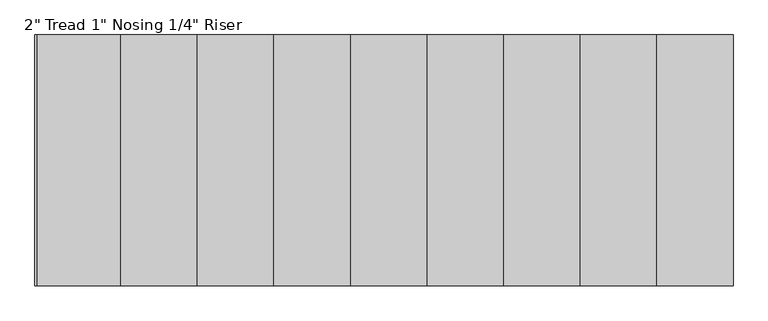
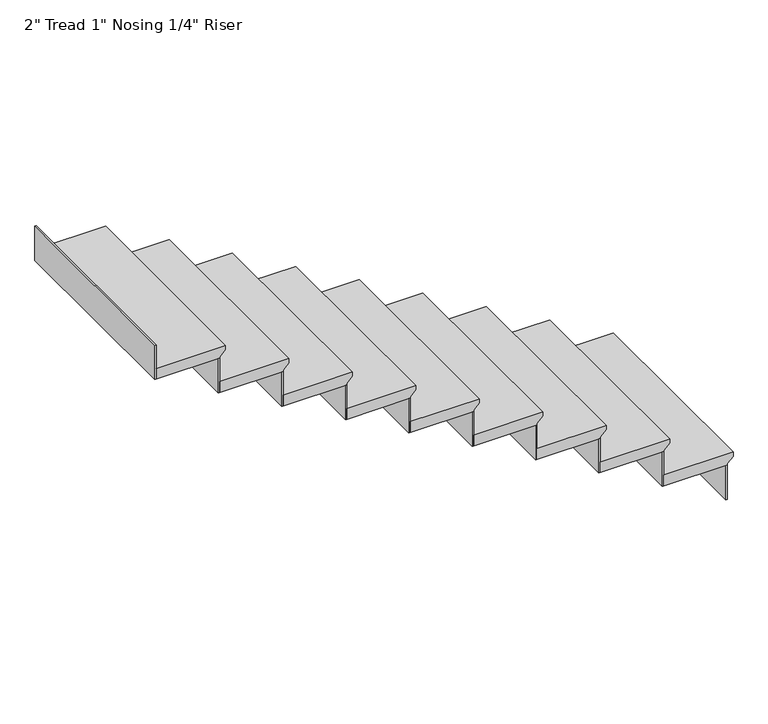
"""IFC4 building model written with IfcOpenShell, lengths in millimetres: stair flight geometry."""

from ifc_helpers import new_model, si_unit, frame, origin, place, context, project, spatial, polyline, outline, extrude, source, transform, mapped, element, save


def stair_flight_f2ac7941(model_context):
    return source(origin(), model_context, "Body", "SweptSolid", [
        extrude(outline(polyline([(20962.62, 923.4845537), (20962.62, 618.6845537), (20911.82, 618.6845537), (20911.82, 898.0845537), (20918.17, 898.0845537), (20943.57, 923.4845537), (20962.62, 923.4845537)])), frame((0.0, -5753.3544725, 0.0), z_axis=(0.0, 1.0, 0.0), x_axis=(0.0, 0.0, 1.0)), (0.0, 0.0, 1.0), 914.4),
        extrude(outline(polyline([(891.7345537, -4838.9544725), (898.0845537, -4838.9544725), (898.0845537, -5753.3544725), (891.7345537, -5753.3544725), (891.7345537, -4838.9544725)])), frame((0.0, 0.0, 20751.8), z_axis=(0.0, 0.0, 1.0), x_axis=(1.0, 0.0, 0.0)), (0.0, 0.0, 1.0), 160.02),
        extrude(outline(polyline([(612.3345537, -4838.9544725), (618.6845537, -4838.9544725), (618.6845537, -5753.3544725), (612.3345537, -5753.3544725), (612.3345537, -4838.9544725)])), frame((0.0, 0.0, 20911.82), z_axis=(0.0, 0.0, 1.0), x_axis=(1.0, 0.0, 0.0)), (0.0, 0.0, 1.0), 160.02),
        extrude(outline(polyline([(21122.64, 644.0845537), (21122.64, 339.2845537), (21071.84, 339.2845537), (21071.84, 618.6845537), (21078.19, 618.6845537), (21103.59, 644.0845537), (21122.64, 644.0845537)])), frame((0.0, -5753.3544725, 0.0), z_axis=(0.0, 1.0, 0.0), x_axis=(0.0, 0.0, 1.0)), (0.0, 0.0, 1.0), 914.4),
        extrude(outline(polyline([(332.9345537, -4838.9544725), (339.2845537, -4838.9544725), (339.2845537, -5753.3544725), (332.9345537, -5753.3544725), (332.9345537, -4838.9544725)])), frame((0.0, 0.0, 21071.84), z_axis=(0.0, 0.0, 1.0), x_axis=(1.0, 0.0, 0.0)), (0.0, 0.0, 1.0), 160.02),
        extrude(outline(polyline([(21282.66, 364.6845537), (21282.66, 59.8845537), (21231.86, 59.8845537), (21231.86, 339.2845537), (21238.21, 339.2845537), (21263.61, 364.6845537), (21282.66, 364.6845537)])), frame((0.0, -5753.3544725, 0.0), z_axis=(0.0, 1.0, 0.0), x_axis=(0.0, 0.0, 1.0)), (0.0, 0.0, 1.0), 914.4),
        extrude(outline(polyline([(53.5345537, -4838.9544725), (59.8845537, -4838.9544725), (59.8845537, -5753.3544725), (53.5345537, -5753.3544725), (53.5345537, -4838.9544725)])), frame((0.0, 0.0, 21231.86), z_axis=(0.0, 0.0, 1.0), x_axis=(1.0, 0.0, 0.0)), (0.0, 0.0, 1.0), 160.02),
        extrude(outline(polyline([(21442.68, 85.2845537), (21442.68, -219.5154463), (21391.88, -219.5154463), (21391.88, 59.8845537), (21398.23, 59.8845537), (21423.63, 85.2845537), (21442.68, 85.2845537)])), frame((0.0, -5753.3544725, 0.0), z_axis=(0.0, 1.0, 0.0), x_axis=(0.0, 0.0, 1.0)), (0.0, 0.0, 1.0), 914.4),
        extrude(outline(polyline([(-225.8654463, -4838.9544725), (-219.5154463, -4838.9544725), (-219.5154463, -5753.3544725), (-225.8654463, -5753.3544725), (-225.8654463, -4838.9544725)])), frame((0.0, 0.0, 21391.88), z_axis=(0.0, 0.0, 1.0), x_axis=(1.0, 0.0, 0.0)), (0.0, 0.0, 1.0), 160.02),
        extrude(outline(polyline([(21602.7, -194.1154463), (21602.7, -498.9154463), (21551.9, -498.9154463), (21551.9, -219.5154463), (21558.25, -219.5154463), (21583.65, -194.1154463), (21602.7, -194.1154463)])), frame((0.0, -5753.3544725, 0.0), z_axis=(0.0, 1.0, 0.0), x_axis=(0.0, 0.0, 1.0)), (0.0, 0.0, 1.0), 914.4),
        extrude(outline(polyline([(-505.2654463, -4838.9544725), (-498.9154463, -4838.9544725), (-498.9154463, -5753.3544725), (-505.2654463, -5753.3544725), (-505.2654463, -4838.9544725)])), frame((0.0, 0.0, 21551.9), z_axis=(0.0, 0.0, 1.0), x_axis=(1.0, 0.0, 0.0)), (0.0, 0.0, 1.0), 160.02),
        extrude(outline(polyline([(21762.72, -473.5154463), (21762.72, -778.3154463), (21711.92, -778.3154463), (21711.92, -498.9154463), (21718.27, -498.9154463), (21743.67, -473.5154463), (21762.72, -473.5154463)])), frame((0.0, -5753.3544725, 0.0), z_axis=(0.0, 1.0, 0.0), x_axis=(0.0, 0.0, 1.0)), (0.0, 0.0, 1.0), 914.4),
        extrude(outline(polyline([(-784.6654463, -4838.9544725), (-778.3154463, -4838.9544725), (-778.3154463, -5753.3544725), (-784.6654463, -5753.3544725), (-784.6654463, -4838.9544725)])), frame((0.0, 0.0, 21711.92), z_axis=(0.0, 0.0, 1.0), x_axis=(1.0, 0.0, 0.0)), (0.0, 0.0, 1.0), 160.02),
        extrude(outline(polyline([(21922.74, -752.9154463), (21922.74, -1057.7154463), (21871.94, -1057.7154463), (21871.94, -778.3154463), (21878.29, -778.3154463), (21903.69, -752.9154463), (21922.74, -752.9154463)])), frame((0.0, -5753.3544725, 0.0), z_axis=(0.0, 1.0, 0.0), x_axis=(0.0, 0.0, 1.0)), (0.0, 0.0, 1.0), 914.4),
        extrude(outline(polyline([(-1064.0654463, -4838.9544725), (-1057.7154463, -4838.9544725), (-1057.7154463, -5753.3544725), (-1064.0654463, -5753.3544725), (-1064.0654463, -4838.9544725)])), frame((0.0, 0.0, 21871.94), z_axis=(0.0, 0.0, 1.0), x_axis=(1.0, 0.0, 0.0)), (0.0, 0.0, 1.0), 160.02),
        extrude(outline(polyline([(22082.76, -1032.3154463), (22082.76, -1337.1154463), (22031.96, -1337.1154463), (22031.96, -1057.7154463), (22038.31, -1057.7154463), (22063.71, -1032.3154463), (22082.76, -1032.3154463)])), frame((0.0, -5753.3544725, 0.0), z_axis=(0.0, 1.0, 0.0), x_axis=(0.0, 0.0, 1.0)), (0.0, 0.0, 1.0), 914.4),
        extrude(outline(polyline([(-1343.4654463, -4838.9544725), (-1337.1154463, -4838.9544725), (-1337.1154463, -5753.3544725), (-1343.4654463, -5753.3544725), (-1343.4654463, -4838.9544725)])), frame((0.0, 0.0, 22031.96), z_axis=(0.0, 0.0, 1.0), x_axis=(1.0, 0.0, 0.0)), (0.0, 0.0, 1.0), 160.02),
        extrude(outline(polyline([(-1622.8654463, -4838.9544725), (-1616.5154463, -4838.9544725), (-1616.5154463, -5753.3544725), (-1622.8654463, -5753.3544725), (-1622.8654463, -4838.9544725)])), frame((0.0, 0.0, 22191.98), z_axis=(0.0, 0.0, 1.0), x_axis=(1.0, 0.0, 0.0)), (0.0, 0.0, 1.0), 160.02),
        extrude(outline(polyline([(22242.78, -1311.7154463), (22242.78, -1616.5154463), (22191.98, -1616.5154463), (22191.98, -1337.1154463), (22198.33, -1337.1154463), (22223.73, -1311.7154463), (22242.78, -1311.7154463)])), frame((0.0, -5753.3544725, 0.0), z_axis=(0.0, 1.0, 0.0), x_axis=(0.0, 0.0, 1.0)), (0.0, 0.0, 1.0), 914.4),
    ])


if __name__ == "__main__":
    model = new_model("IFC4")
    model_context = context("Model", 3, world=origin())
    ifc_project = project(units=[si_unit("LENGTHUNIT", "METRE", prefix="MILLI")], contexts=[model_context])
    site = spatial("IfcSite", under=ifc_project)
    building = spatial("IfcBuilding", under=site)
    placement = place(None, origin())
    stair_flight_shape = stair_flight_f2ac7941(model_context)
    element("IfcStairFlight", 1, ObjectType="2\" Tread 1\" Nosing 1/4\" Riser", at=placement, inside=building, context=model_context, shape_type="MappedRepresentation", body=[
        mapped(stair_flight_shape, transform((0.0, 0.0, 0.0), x_axis=(1.0, 0.0, 0.0), y_axis=(0.0, 1.0, 0.0), z_axis=(0.0, 0.0, 1.0))),
    ])
    save(model, "model.ifc")
